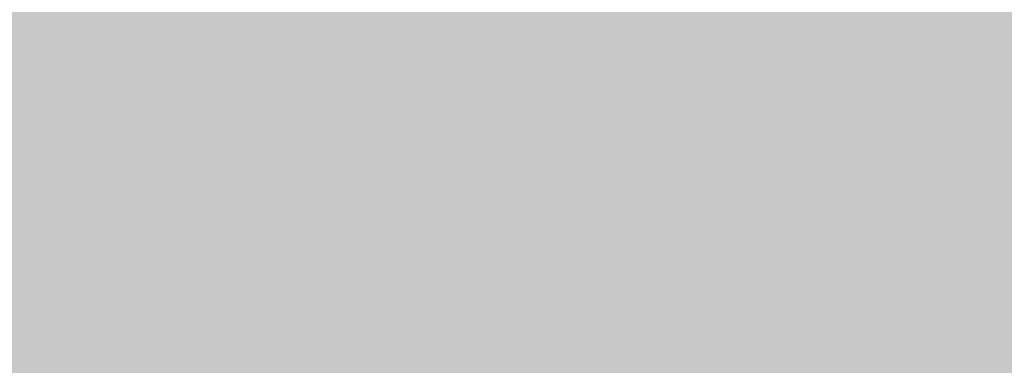
# Model space of a CAD drawing. Units: inches. Extents: x 2091 to 2899, y 967 to 2217.
# Tile 188 of 256: x 2203.16122 to 2203.18039, y 1152.25378 to 1152.26051. Entities that reach past the tile are written whole.
import ezdxf

# ---------------------------------------------------------------- set-up
doc = ezdxf.new("R2010")
doc.units = ezdxf.units.IN
doc.layers.add('A-WALL-PATT', color=141, linetype='Continuous', lineweight=13, true_color=0xadddf7)

msp = doc.modelspace()

# ---------------------------------------------------------------- hatches: boundary and pattern name
at = {"layer": 'A-WALL-PATT'}
h = msp.add_hatch(color=256, dxfattribs=at)
h.dxf.hatch_style = 1
h.paths.add_polyline_path([(2803.143603, 2050.919059), (2203.143603, 2050.919059), (2203.143603, 1090.919059), (2803.143603, 1090.919059)])
h.paths.add_polyline_path([(2635.79885, 1147.540465), (2674.524052, 1147.540465, 0.376086), (2678.529665, 1152.880202), (2678.529665, 1159.556473, 0.333335), (2674.524319, 1163.561846), (2674.524319, 1163.56185), (2674.524319, 1192.93439), (2635.805971, 1192.93439), (2597.087622, 1192.93439), (2597.087622, 1163.561846, 0.333335), (2593.082276, 1159.556473), (2593.082276, 1152.880202, 0.376086), (2597.087889, 1147.540465)], flags=0)
h.paths.add_polyline_path([(2436.010433, 1278.240778, 0.000483), (2435.952643, 1278.215027, -0.001328), (2435.935625, 1278.111693, -0.001711), (2436.11644, 1278.040758, 0.002185)], flags=0)
h.paths.add_polyline_path([(2794.143603, 1143.419059), (2794.143603, 1347.419059), (2543.370171, 1347.419059), (2543.370171, 1351.919059), (2794.143603, 1351.919059), (2794.143603, 1392.713555), (2793.947398, 1392.713555), (2793.947398, 1473.5369), (2794.143603, 1473.5369), (2794.143603, 1531.919059), (2650.143603, 1531.919059), (2650.143603, 1536.419059), (2794.143603, 1536.419059), (2794.143603, 1692.419059), (2609.375609, 1692.419059), (2609.375609, 1644.419059), (2604.875609, 1644.419059), (2604.875609, 1744.919059), (2609.375609, 1744.919059), (2609.375609, 1696.919059), (2794.143603, 1696.919059), (2794.143603, 1780.919059), (2609.643603, 1780.919059), (2493.875609, 1780.919059), (2493.875609, 1785.419059), (2609.643603, 1785.419059), (2794.143603, 1785.419059), (2794.143603, 1847.938821), (2793.951222, 1847.938821), (2793.951222, 1928.762166), (2794.143603, 1928.762166), (2794.143603, 1941.419059), (2614.143603, 1941.419059), (2614.143603, 1821.419059), (2609.643603, 1821.419059), (2609.643603, 1941.419059), (2392.143603, 1941.419059), (2392.143603, 1819.919059), (2387.643603, 1819.919059), (2387.643603, 1941.419059), (2212.143603, 1941.419059), (2212.143603, 1783.919059), (2392.143603, 1783.919059), (2392.143603, 1780.919059), (2212.143603, 1780.919059), (2212.143603, 1629.419059), (2387.643603, 1629.419059), (2387.643603, 1744.919059), (2392.143603, 1744.919059), (2392.143603, 1627.919059), (2317.143603, 1627.919059), (2317.143603, 1551.419059), (2317.143603, 1536.419059), (2459.383591, 1536.419059), (2459.383591, 1602.39648), (2463.883591, 1602.39648), (2463.883591, 1531.919059), (2456.643603, 1531.919059), (2456.643603, 1529.919059), (2452.143603, 1529.919059), (2452.143603, 1531.919059), (2312.643603, 1531.919059), (2312.643603, 1551.419059), (2306.143603, 1551.419059), (2306.143603, 1555.919059), (2308.143603, 1555.919059), (2308.143603, 1551.419059), (2312.643603, 1551.419059), (2312.643603, 1627.919059), (2212.143603, 1627.919059), (2212.143603, 1555.919059), (2270.143603, 1555.919059), (2270.143603, 1551.419059), (2212.143603, 1551.419059), (2212.143603, 1351.919059), (2272.143603, 1351.919059), (2272.143603, 1347.419059), (2212.143603, 1347.419059), (2212.143603, 1275.419059), (2308.143603, 1275.419059), (2308.143603, 1351.919059), (2452.143603, 1351.919059), (2452.143603, 1493.919059), (2456.643603, 1493.919059), (2456.643603, 1347.419059), (2312.643603, 1347.419059), (2312.643603, 1270.919059), (2212.143603, 1270.919059), (2212.143603, 1099.919059), (2281.237523, 1099.919059), (2282.871041, 1110.913803), (2282.008341, 1116.996603), (2278.557741, 1121.420403), (2268.205641, 1128.056203), (2272.087641, 1128.056203), (2273.812941, 1131.927003), (2279.420341, 1134.691903), (2285.027841, 1135.244903), (2287.615841, 1137.456803), (2288.047141, 1138.009803), (2289.341141, 1140.774703), (2291.066541, 1139.668703), (2292.360541, 1135.244903), (2295.379841, 1136.903803), (2296.242541, 1135.797903), (2297.105241, 1133.033003), (2300.124641, 1138.009803), (2303.143941, 1138.009803), (2304.437941, 1135.797903), (2303.143941, 1133.586003), (2306.594641, 1134.691903), (2307.888741, 1133.033003), (2310.908041, 1135.244903), (2313.927441, 1134.138903), (2315.62686, 1132.427102), (2308.320041, 1117.549603), (2290.203841, 1109.807903), (2288.909841, 1103.172103), (2289.272309, 1099.919059), (2434.918227, 1099.919059), (2431.593227, 1124.788059), (2429.930227, 1169.553059), (2430.927185, 1240.519694), (2435.658926, 1238.186126), (2437.135227, 1196.554059), (2438.798227, 1143.973059), (2442.678227, 1111.998059), (2446.558227, 1099.919059), (2794.143603, 1099.919059), (2794.143603, 1138.919059), (2548.032447, 1138.919059), (2548.032447, 1143.419059), (2548.032447, 1148.819059), (2546.668457, 1148.031559), (2528.685692, 1179.178622, 0.256256), (2512.032447, 1148.819059), (2512.032447, 1143.419059), (2512.032447, 1138.919059), (2507.532447, 1138.919059), (2507.532447, 1143.419059), (2507.532447, 1148.819059, 0.256256), (2490.879202, 1179.178622), (2472.896437, 1148.031559), (2471.532447, 1148.819059), (2471.532447, 1143.419059), (2467.032447, 1143.419059), (2467.032447, 1269.945786, 0.039061), (2460.909987, 1273.580059), (2467.032447, 1273.580059), (2467.032447, 1286.325364, 0.014511), (2465.216194, 1286.761905), (2467.032447, 1287.052576), (2467.032447, 1323.419059), (2471.532447, 1323.419059), (2471.532447, 1148.819059), (2489.532447, 1179.995973), (2490.896437, 1179.208473), (2490.879202, 1179.178622, -0.256256), (2507.532447, 1148.819059), (2507.532447, 1143.419059), (2512.032447, 1143.419059), (2512.032447, 1148.819059, -0.256256), (2528.685692, 1179.178622), (2528.668457, 1179.208473), (2530.032447, 1179.995973), (2548.032447, 1148.819059), (2548.032447, 1143.419059)], flags=16)
h.paths.add_polyline_path([(2607.768546, 1200.945083), (2607.768546, 1265.030625), (2597.087622, 1281.052011), (2619.784585, 1281.052011), (2627.795278, 1337.12686), (2635.79885, 1337.12686), (2643.816663, 1337.12686), (2651.827356, 1281.052011), (2674.524319, 1281.052011), (2663.843395, 1265.030625), (2663.843395, 1200.945083), (2635.805971, 1200.945083)], flags=0)
edge = h.paths.add_edge_path(flags=0)
edge.add_ellipse((13303.896215, 1272.998725), major_axis=(-10595.31304, 0.000001), ratio=0.842303870086, start_angle=0.6282372191, end_angle=0.6465540999, ccw=False)
edge.add_ellipse((2711.70045, 1156.852678), major_axis=(2.219769, 0), ratio=0.84230387, start_angle=111.535244, end_angle=180.628237, ccw=False)
edge.add_ellipse((13303.156292, 1272.998725), major_axis=(-10593.026306, 0), ratio=0.842303869544, start_angle=0.5282714718, end_angle=0.6465540971, ccw=False)
edge.add_line((2710.764596, 1175.333295), (2710.129986, 1175.333295))
edge.add_ellipse((2710.129986, 1176.579775), major_axis=(1.479846, 0), ratio=0.84230387, start_angle=180, end_angle=270, ccw=False)
edge.add_line((2708.65014, 1176.579775), (2708.65014, 1200.782914))
edge.add_ellipse((2710.129986, 1200.782914), major_axis=(1.479846, 0), ratio=0.84230387, start_angle=90, end_angle=180, ccw=False)
edge.add_line((2710.129986, 1202.029394), (2710.465075, 1202.029394))
edge.add_ellipse((13303.156292, 1272.998725), major_axis=(-10593.026306, 0), ratio=0.842303869544, start_angle=-0.0902290886, end_angle=0.3838667788, ccw=False)
edge.add_ellipse((2710.129986, 1290.927031), major_axis=(-1.479846, 0), ratio=0.84230387, start_angle=0, end_angle=90, ccw=False)
edge.add_line((2708.65014, 1290.927031), (2708.65014, 1315.13017))
edge.add_ellipse((2710.129986, 1315.13017), major_axis=(-1.479846, 0), ratio=0.84230387, start_angle=-90, end_angle=0, ccw=False)
edge.add_line((2710.129986, 1316.37665), (2710.706314, 1316.37665))
edge.add_ellipse((3238.40172, 1296.289566), major_axis=(528.234, 0), ratio=0.8423038695, start_angle=176.34957241, end_angle=177.82004969, ccw=False)
edge.add_ellipse((2775.063043, 1071.450696), major_axis=(313.307761, 0), ratio=0.8423038695, start_angle=102.12596555, end_angle=103.78052899, ccw=False)
edge.add_ellipse((2775.063043, 1078.305698), major_axis=(-305.302891, 0), ratio=0.8423038695, start_angle=-79.790461, end_angle=-77.55537271, ccw=False)
edge.add_ellipse((2695.141767, 1541.975383), major_axis=(-250.960216, 0), ratio=0.8423038695, start_angle=99.25656601, end_angle=102.55493264)
edge.add_line((2741.410326, 1334.214255), (2747.132545, 1337.378477))
edge.add_ellipse((2747.538616, 1336.857478), major_axis=(-0.739923, 0), ratio=0.8423039, start_angle=270, end_angle=307.93313, ccw=False)
edge.add_ellipse((2747.538616, 1336.857478), major_axis=(-0.739923, 0), ratio=0.8423039, start_angle=232.06687, end_angle=270, ccw=False)
edge.add_line((2747.944687, 1337.378477), (2753.666906, 1334.214255))
edge.add_ellipse((2799.935466, 1541.975383), major_axis=(250.960216, 0), ratio=0.8423038695, start_angle=257.44506736, end_angle=260.74343399)
edge.add_ellipse((2720.014189, 1078.305698), major_axis=(305.302891, 0), ratio=0.8423038695, start_angle=77.55537271, end_angle=79.790461, ccw=False)
edge.add_ellipse((2720.014189, 1071.450696), major_axis=(-313.307761, 0), ratio=0.8423038695, start_angle=256.21947101, end_angle=257.87403445, ccw=False)
edge.add_ellipse((2256.675512, 1296.289566), major_axis=(-528.234, 0), ratio=0.8423038695, start_angle=182.17995031, end_angle=183.65042759, ccw=False)
edge.add_line((2784.370918, 1316.37665), (2784.947247, 1316.37665))
edge.add_ellipse((2784.947247, 1315.13017), major_axis=(1.479846, 0), ratio=0.84230387, start_angle=0, end_angle=90, ccw=False)
edge.add_line((2786.427093, 1315.13017), (2786.427093, 1290.927031))
edge.add_ellipse((2784.947247, 1290.927031), major_axis=(1.479846, 0), ratio=0.84230387, start_angle=270, end_angle=360, ccw=False)
edge.add_ellipse((-7808.07906, 1272.998725), major_axis=(10593.026306, 0), ratio=0.842303869544, start_angle=-0.3838667788, end_angle=0.0902290886, ccw=False)
edge.add_line((2784.612157, 1202.029394), (2784.947247, 1202.029394))
edge.add_ellipse((2784.947247, 1200.782914), major_axis=(1.479846, 0), ratio=0.84230387, start_angle=0, end_angle=90, ccw=False)
edge.add_line((2786.427093, 1200.782914), (2786.427093, 1176.579775))
edge.add_ellipse((2784.947247, 1176.579775), major_axis=(-1.479846, 0), ratio=0.84230387, start_angle=90, end_angle=180, ccw=False)
edge.add_line((2784.947247, 1175.333295), (2784.312636, 1175.333295))
edge.add_ellipse((-7808.07906, 1272.998725), major_axis=(10593.026306, 0), ratio=0.842303869544, start_angle=-0.6186431963, end_angle=-0.5282714718, ccw=False)
edge.add_ellipse((2783.376783, 1156.852678), major_axis=(-2.219769, 0), ratio=0.84230387, start_angle=179.371763, end_angle=248.464757, ccw=False)
edge.add_ellipse((-7808.818983, 1272.998725), major_axis=(-10595.31304, 0.000004), ratio=0.842303865762, start_angle=179.3534459226, end_angle=179.3717628034, ccw=False)
edge.add_ellipse((2780.297303, 1153.500793), major_axis=(-5.246426, 0), ratio=0.84230387, start_angle=90, end_angle=179.353446, ccw=False)
edge.add_line((2780.297303, 1149.081708), (2714.77993, 1149.081708))
edge.add_ellipse((2714.77993, 1153.500793), major_axis=(5.246426, 0), ratio=0.84230387, start_angle=180.646554, end_angle=270, ccw=False)
edge = h.paths.add_edge_path(flags=0)
edge.add_line((2718.187367, 1151.007833), (2718.187367, 1170.472364))
edge.add_ellipse((2721.14706, 1170.472364), major_axis=(-2.959692, 0), ratio=0.84230387, start_angle=-90, end_angle=0, ccw=False)
edge.add_line((2721.14706, 1172.965324), (2773.930173, 1172.965324))
edge.add_ellipse((2773.930173, 1170.472364), major_axis=(-2.959692, 0), ratio=0.84230387, start_angle=180, end_angle=270, ccw=False)
edge.add_line((2776.889865, 1170.472364), (2776.889865, 1151.007833))
edge.add_line((2776.889865, 1151.007833), (2718.187367, 1151.007833))
edge = h.paths.add_edge_path(flags=0)
edge.add_line((2718.187367, 1180.23415), (2718.187367, 1199.057834))
edge.add_ellipse((2747.538616, 1320.39864), major_axis=(147.017924, 0), ratio=0.8423038695, start_angle=256.40186531, end_angle=283.59813469)
edge.add_line((2776.889865, 1199.057834), (2776.889865, 1180.23415))
edge.add_ellipse((2747.538616, 1301.574956), major_axis=(147.017924, 0), ratio=0.8423038695, start_angle=256.40186531, end_angle=283.59813469, ccw=False)
edge = h.paths.add_edge_path(flags=0)
edge.add_ellipse((13303.156292, 1272.998725), major_axis=(-10591.54646, 0), ratio=0.842303869555, start_angle=0.0555943135, end_angle=0.3777641939, ccw=False)
edge.add_line((2711.616859, 1262.72171), (2715.667408, 1249.495396))
edge.add_ellipse((6413.891963, 1241.691919), major_axis=(-3698.236159, 0), ratio=0.84230386955, start_angle=-0.120897369, end_angle=0.364076349)
edge.add_line((2715.761038, 1218.192455), (2711.934307, 1203.167361))
edge = h.paths.add_edge_path(flags=0)
edge.add_line((2718.187367, 1251.074566), (2716.002485, 1267.450435))
edge.add_ellipse((2742.151175, 1202.18954), major_axis=(81.772585, 0), ratio=0.84230387, start_angle=94.27742096, end_angle=111.8349538, ccw=False)
edge.add_line((2737.009748, 1270.930626), (2758.067484, 1270.930626))
edge.add_ellipse((2752.926058, 1202.18954), major_axis=(81.772585, 0), ratio=0.84230387, start_angle=68.1650462, end_angle=85.72257904, ccw=False)
edge.add_line((2779.074747, 1267.450435), (2776.889865, 1251.074566))
edge.add_ellipse((2750.338059, 1187.885356), major_axis=(79.579664, 0), ratio=0.84230387, start_angle=67.20808512, end_angle=85.1299304)
edge.add_line((2756.034656, 1254.743656), (2739.042576, 1254.743656))
edge.add_ellipse((2744.739174, 1187.885356), major_axis=(79.579664, 0), ratio=0.84230387, start_angle=94.8700696, end_angle=112.79191488)
edge = h.paths.add_edge_path(flags=0)
edge.add_line((2783.142926, 1203.167361), (2779.316194, 1218.192455))
edge.add_ellipse((-918.81473, 1241.691919), major_axis=(3698.236159, 0), ratio=0.84230386955, start_angle=-0.364076349, end_angle=0.120897369)
edge.add_line((2779.409825, 1249.495396), (2783.460373, 1262.72171))
edge.add_ellipse((-7808.07906, 1272.998725), major_axis=(-10591.54646, 0), ratio=0.84230386954, start_angle=179.6222358061, end_angle=179.9444056865, ccw=False)
edge = h.paths.add_edge_path(flags=0)
edge.add_ellipse((2734.200892, 1286.69044), major_axis=(-0.356609, 6.340078), ratio=0.60383358, start_angle=89.0020143, end_angle=253.657408, ccw=False)
edge.add_line((2730.369001, 1286.541806), (2730.369001, 1301.35198))
edge.add_line((2730.369001, 1301.35198), (2735.913311, 1305.214803))
edge.add_ellipse((2736.384917, 1304.734561), major_axis=(0.739923, 0), ratio=0.8423039, start_angle=90, end_angle=134.480211, ccw=False)
edge.add_line((2736.384917, 1305.357801), (2738.032783, 1305.357801))
edge.add_line((2738.032783, 1305.357801), (2738.032783, 1307.707927))
edge.add_ellipse((2794.201642, 1307.707927), major_axis=(56.168859, 0), ratio=0.84230387, start_angle=150.5614304, end_angle=180, ccw=False)
edge.add_ellipse((2700.875591, 1307.707927), major_axis=(-56.168859, 0), ratio=0.84230387, start_angle=180, end_angle=209.4385696, ccw=False)
edge.add_line((2757.04445, 1307.707927), (2757.04445, 1305.357801))
edge.add_line((2757.04445, 1305.357801), (2758.692316, 1305.357801))
edge.add_ellipse((2758.692316, 1304.734561), major_axis=(-0.739923, 0), ratio=0.8423039, start_angle=225.519789, end_angle=270, ccw=False)
edge.add_line((2759.163922, 1305.214803), (2764.708231, 1301.35198))
edge.add_line((2764.708231, 1301.35198), (2764.708231, 1286.541806))
edge.add_ellipse((2760.87634, 1286.69044), major_axis=(0.356609, 6.340078), ratio=0.60383358, start_angle=106.342592, end_angle=270.9979857, ccw=False)
edge.add_line((2757.04445, 1285.79709), (2757.04445, 1307.707927))
edge.add_ellipse((2700.875591, 1307.707927), major_axis=(-56.168859, 0), ratio=0.84230387, start_angle=180, end_angle=209.4385696)
edge.add_ellipse((2794.201642, 1307.707927), major_axis=(56.168859, 0), ratio=0.84230387, start_angle=150.5614304, end_angle=180)
edge.add_line((2738.032783, 1307.707927), (2738.032783, 1285.79709))
h.paths.add_polyline_path([(2417.812273, 1104.449704), (2413.492273, 1102.529704), (2410.612273, 1103.969704), (2409.172273, 1106.369704), (2407.252273, 1107.329704), (2406.292273, 1109.729704), (2405.332273, 1114.049704), (2405.332273, 1117.889704), (2406.292273, 1120.129704), (2407.252273, 1119.809704), (2408.848322, 1118.327658), (2410.173945, 1119.42417), (2410.211273, 1120.405704), (2411.040731, 1121.419054), (2410.699273, 1119.858704), (2410.173945, 1119.42417), (2410.088452, 1117.176109), (2411.132836, 1116.206324), (2413.972273, 1119.329704), (2416.852273, 1120.769704), (2416.869721, 1120.798784), (2417.035071, 1119.405116), (2417.896213, 1118.143384), (2418.292273, 1118.369704), (2419.544447, 1120.039269), (2419.360915, 1118.387487), (2419.032108, 1119.356151), (2418.398939, 1118.511926), (2419.252273, 1114.529704), (2418.794091, 1107.198795)], flags=0)
h.paths.add_polyline_path([(2508.870171, 1347.419059), (2508.370171, 1347.419059), (2508.370171, 1351.919059), (2508.870171, 1351.919059)], flags=0)
h.paths.add_polyline_path([(2473.370171, 1347.419059), (2472.370171, 1347.419059), (2467.870171, 1347.419059), (2467.870171, 1455.419059), (2472.370171, 1455.419059), (2472.370171, 1352.419059), (2473.370171, 1352.419059)], flags=0)
h.paths.add_polyline_path([(2352.106244, 1217.446197), (2349.226244, 1218.886197), (2347.786244, 1221.286197), (2345.866244, 1222.246197), (2344.906244, 1224.646197), (2343.946244, 1228.966197), (2343.946244, 1232.806197), (2344.906244, 1235.046197), (2345.866244, 1234.726197), (2347.462293, 1233.244152), (2348.787916, 1234.340663), (2348.825244, 1235.322197), (2349.654702, 1236.335547), (2349.313244, 1234.775197), (2348.787916, 1234.340663), (2348.702423, 1232.092603), (2349.746807, 1231.122817), (2352.586244, 1234.246197), (2355.466244, 1235.686197), (2355.483692, 1235.715277), (2355.649043, 1234.321609), (2356.510185, 1233.059877), (2356.906244, 1233.286197), (2358.158418, 1234.955762), (2357.974887, 1233.30398), (2357.646079, 1234.272644), (2357.012911, 1233.428419), (2357.866244, 1229.446197), (2357.408062, 1222.115288), (2356.426244, 1219.366197)], flags=0)
h.paths.add_polyline_path([(2348.2968, 1112.22442), (2347.0138, 1112.31042), (2345.5298, 1114.12742), (2345.7318, 1115.85842), (2346.8118, 1116.98242), (2346.8118, 1114.64642), (2345.8668, 1114.21442), (2346.8798, 1114.30042)], flags=0)
h.paths.add_polyline_path([(2347.0138, 1110.92642), (2346.2718, 1110.49342), (2346.6098, 1111.18642)], flags=0)
h.paths.add_polyline_path([(2345.8668, 1118.19442), (2345.5298, 1117.32942), (2343.7078, 1118.02142), (2344.3828, 1118.62642)], flags=0)
h.paths.add_polyline_path([(2346.6768, 1109.28242), (2346.0698, 1108.07142), (2345.8668, 1110.06142)], flags=0)
h.paths.add_polyline_path([(2345.0568, 1119.75142), (2343.6398, 1119.75142), (2343.9778, 1121.13542)], flags=0)
h.paths.add_polyline_path([(2345.2598, 1116.55042), (2345.1248, 1115.85842), (2344.9218, 1115.68542), (2344.7198, 1116.37742)], flags=0)
h.paths.add_polyline_path([(2345.6648, 1112.31042), (2345.4618, 1111.53242), (2344.0448, 1111.96442), (2344.6518, 1112.57042)], flags=0)
h.paths.add_polyline_path([(2345.1918, 1113.34942), (2344.4498, 1113.86842), (2344.7198, 1114.38742)], flags=0)
h.paths.add_polyline_path([(2344.6518, 1116.80942), (2344.1798, 1115.68542), (2344.6518, 1115.33942), (2343.9098, 1114.90642), (2343.0328, 1115.94442), (2343.6398, 1116.46342)], flags=0)
h.paths.add_polyline_path([(2345.8668, 1106.68642), (2344.9898, 1105.56242), (2344.5168, 1106.60042)], flags=0)
h.paths.add_polyline_path([(2344.8548, 1110.06142), (2344.5168, 1109.28242), (2344.1128, 1109.71542)], flags=0)
h.paths.add_polyline_path([(2344.0448, 1113.52242), (2343.4378, 1113.08942), (2342.7628, 1113.95442)], flags=0)
h.paths.add_polyline_path([(2344.3148, 1111.01242), (2342.9648, 1110.32042), (2342.9648, 1111.09942)], flags=0)
h.paths.add_polyline_path([(2345.1248, 1104.69742), (2344.5848, 1103.74542), (2344.4498, 1104.26442)], flags=0)
h.paths.add_polyline_path([(2342.8298, 1121.22242), (2341.7498, 1120.53042), (2340.5358, 1121.04942), (2340.1308, 1121.82842), (2340.6708, 1122.95242), (2341.1428, 1121.82842), (2341.6148, 1122.00142)], flags=0)
h.paths.add_polyline_path([(2342.9648, 1119.75142), (2343.0328, 1118.45342), (2342.0878, 1118.02142), (2342.0198, 1119.49142)], flags=0)
h.paths.add_polyline_path([(2342.6948, 1116.89642), (2341.9528, 1116.63642), (2342.0198, 1117.32942)], flags=0)
h.paths.add_polyline_path([(2343.0328, 1112.22442), (2342.0198, 1111.79142), (2341.5478, 1112.22442), (2342.3578, 1113.34942)], flags=0)
h.paths.add_polyline_path([(2343.7748, 1104.43742), (2342.6278, 1102.88042), (2342.6948, 1104.61042), (2343.4378, 1105.12942)], flags=0)
h.paths.add_polyline_path([(2342.0198, 1115.07942), (2340.8058, 1115.51242), (2340.9408, 1116.37742)], flags=0)
h.paths.add_polyline_path([(2341.4808, 1120.09742), (2341.4808, 1119.40542), (2341.0758, 1119.57842), (2341.1428, 1120.09742)], flags=0)
h.paths.add_polyline_path([(2341.8178, 1114.47342), (2340.9408, 1113.08942), (2340.8058, 1114.56042)], flags=0)
h.paths.add_polyline_path([(2341.1428, 1118.54042), (2340.9408, 1116.98242), (2339.0508, 1117.67542), (2339.0508, 1118.62642)], flags=0)
h.paths.add_polyline_path([(2342.6948, 1101.66842), (2341.9528, 1101.84142), (2342.5598, 1102.36142)], flags=0)
h.paths.add_polyline_path([(2340.3328, 1119.66542), (2338.4438, 1119.57842), (2337.9038, 1120.35742), (2339.6578, 1120.61642)], flags=0)
h.paths.add_polyline_path([(2340.3328, 1115.33942), (2340.0628, 1113.69542), (2339.3878, 1115.33942)], flags=0)
h.paths.add_polyline_path([(2341.8178, 1103.83142), (2341.5478, 1102.88042), (2341.1428, 1103.65842)], flags=0)
h.paths.add_polyline_path([(2339.0508, 1122.86642), (2337.2958, 1121.82842), (2337.0938, 1123.12542), (2337.7688, 1123.81842)], flags=0)
h.paths.add_polyline_path([(2339.1178, 1121.74142), (2338.8478, 1121.22242), (2338.1738, 1121.04942), (2338.3758, 1121.56842)], flags=0)
h.paths.add_polyline_path([(2339.1858, 1119.31942), (2338.6458, 1118.71342), (2338.2408, 1118.10742), (2338.2408, 1118.88642)], flags=0)
h.paths.add_polyline_path([(2341.1428, 1101.92842), (2340.6028, 1101.23642), (2340.0628, 1101.84142), (2340.6028, 1102.36142)], flags=0)
h.paths.add_polyline_path([(2337.6338, 1117.76142), (2336.6208, 1118.28042), (2337.2958, 1118.97242)], flags=0)
h.paths.add_polyline_path([(2336.8238, 1119.57842), (2334.7988, 1118.97242), (2335.2038, 1120.35742), (2336.5538, 1120.87642)], flags=0)
h.paths.add_polyline_path([(2339.1178, 1100.45742), (2337.3638, 1100.54342), (2336.7558, 1101.23642)], flags=0)
h.paths.add_polyline_path([(2336.3508, 1122.43342), (2336.0138, 1121.91442), (2334.9338, 1122.43342), (2334.5288, 1123.47142), (2335.7438, 1122.77942)], flags=0)
h.paths.add_polyline_path([(2334.7318, 1120.87642), (2334.2588, 1120.35742), (2334.0568, 1120.78942), (2334.5968, 1121.30842)], flags=0)
h.paths.add_polyline_path([(2334.4618, 1122.17442), (2332.5718, 1121.30842), (2331.3568, 1122.17442), (2332.0998, 1122.86642)], flags=0)
h.paths.add_polyline_path([(2334.2588, 1118.54042), (2333.3818, 1118.45342), (2333.6518, 1119.31942)], flags=0)
h.paths.add_polyline_path([(2335.5418, 1102.27442), (2334.1918, 1102.62042), (2335.2718, 1103.31242)], flags=0)
h.paths.add_polyline_path([(2332.7068, 1119.66542), (2331.6948, 1120.44342), (2332.5048, 1120.78942)], flags=0)
h.paths.add_polyline_path([(2334.7318, 1101.14942), (2333.5168, 1101.58242), (2333.9888, 1101.75542)], flags=0)
h.paths.add_polyline_path([(2332.6398, 1116.63642), (2331.0868, 1116.29042), (2331.9648, 1118.19442)], flags=0)
h.paths.add_polyline_path([(2330.7498, 1121.56842), (2330.2768, 1120.27042), (2328.5228, 1119.31942), (2328.9948, 1121.04942)], flags=0)
h.paths.add_polyline_path([(2330.7498, 1118.62642), (2330.0078, 1117.50242), (2329.8728, 1118.02142)], flags=0)
h.paths.add_polyline_path([(2332.0998, 1102.36142), (2330.5468, 1102.01442), (2331.6948, 1102.96642)], flags=0)
h.paths.add_polyline_path([(2329.5348, 1113.60842), (2329.0628, 1112.31042), (2328.5898, 1113.34942)], flags=0)
h.paths.add_polyline_path([(2328.3878, 1117.84842), (2327.5098, 1116.55042), (2327.1728, 1117.76142)], flags=0)
h.paths.add_polyline_path([(2329.7378, 1106.51342), (2329.5348, 1105.30242), (2328.2528, 1106.08142)], flags=0)
h.paths.add_polyline_path([(2328.6578, 1114.38742), (2328.0498, 1114.12742), (2328.3198, 1114.90642)], flags=0)
h.paths.add_polyline_path([(2328.3198, 1112.22442), (2327.1058, 1112.13742), (2326.7008, 1112.65642)], flags=0)
h.paths.add_polyline_path([(2326.9028, 1115.25242), (2326.7008, 1114.12742), (2325.2158, 1113.60842), (2326.0928, 1115.33942)], flags=0)
h.paths.add_polyline_path([(2326.6328, 1108.33042), (2326.0928, 1107.37942), (2325.8908, 1108.50342), (2326.4978, 1109.10942)], flags=0)
h.paths.add_polyline_path([(2615.143603, 1531.919059), (2609.643603, 1531.919059), (2609.643603, 1620.419059), (2614.143603, 1620.419059), (2614.143603, 1536.419059), (2615.143603, 1536.419059)], flags=0)
h.paths.add_polyline_path([(2545.143603, 1563.419059), (2464.143603, 1563.419059), (2464.143603, 1632.419059), (2509.143603, 1632.419059), (2509.143603, 1627.919059), (2509.143603, 1603.919059), (2468.643603, 1603.919059), (2468.643603, 1567.919059), (2540.643603, 1567.919059), (2540.643603, 1591.919059), (2545.143603, 1591.919059)], flags=0)
h.paths.add_polyline_path([(2388.969048, 1549.985735), (2357.434181, 1549.985735), (2357.434181, 1623.360778), (2399.362777, 1623.360778), (2435.689465, 1623.360778), (2435.592547, 1602.559273), (2435.592547, 1602.39648), (2388.969048, 1602.39648)], flags=0)
h.paths.add_polyline_path([(2388.880628, 1555.809151), (2374.904429, 1555.809151), (2374.904429, 1600.571564), (2374.904429, 1615.457645), (2406.350877, 1615.457645), (2406.350877, 1618.939431), (2412.174293, 1615.457645), (2406.350877, 1611.97586), (2406.350877, 1615.457645), (2388.880628, 1615.457645)], flags=0)
h.paths.add_polyline_path([(2568.875609, 1644.419059), (2453.375609, 1644.419059), (2453.375609, 1785.419059), (2457.875609, 1785.419059), (2457.875609, 1648.919059), (2568.875609, 1648.919059)], flags=0)
h.paths.add_polyline_path([(2212.143603, 1945.919059), (2212.143603, 2041.919059), (2794.143603, 2041.919059), (2794.143603, 1945.919059)], flags=16)
h.paths.add_polyline_path([(2271.082728, 1964.317238), (2776.852968, 1964.317238), (2776.852968, 2037.169623), (2271.082728, 2037.169623)], flags=8)
h.paths.add_polyline_path([(2380.649285, 1536.824144), (2461.040809, 1536.824144), (2461.040809, 1554.652587), (2380.649285, 1554.652587)], flags=8)
h.paths.add_polyline_path([(2240.755709, 1609.725451), (2309.185829, 1609.725451), (2309.185829, 1617.698204), (2240.755709, 1617.698204)], flags=8)
h.paths.add_polyline_path([(2212.677255, 1313.504102), (2282.59152, 1313.504102), (2282.59152, 1322.745239), (2212.677255, 1322.745239)], flags=8)
h.paths.add_polyline_path([(2457.111976, 1114.778574), (2558.481581, 1114.778574), (2558.481581, 1142.219682), (2457.111976, 1142.219682)], flags=8)
h.paths.add_polyline_path([(2473.442337, 1273.010067), (2604.641226, 1273.010067), (2604.641226, 1318.346935), (2473.442337, 1318.346935)], flags=8)
h.paths.add_polyline_path([(2638.876302, 1626.977432), (2684.250367, 1627.976738), (2684.038483, 1637.597494), (2638.664417, 1636.598188)], flags=8)
h.paths.add_polyline_path([(2537.590554, 1453.793447), (2628.389547, 1453.793447), (2628.389547, 1475.344811), (2537.590554, 1475.344811)], flags=8)
h.paths.add_polyline_path([(2504.137638, 1714.632397), (2554.647187, 1714.632397), (2554.647187, 1730.237712), (2504.137638, 1730.237712)], flags=8)
h.paths.add_polyline_path([(2487.501181, 1575.651872), (2535.097121, 1575.651872), (2535.097121, 1598.377646), (2487.501181, 1598.377646)], flags=8)
h.paths.add_polyline_path([(2709.0994, 1735.710278), (2740.016601, 1735.710278), (2740.016601, 1749.937641), (2709.0994, 1749.937641)], flags=8)
h.paths.add_polyline_path([(2442.438424, 1792.171657), (2564.728835, 1792.171657), (2564.728835, 1842.000163), (2442.438424, 1842.000163)], flags=8)
h.paths.add_polyline_path([(2655.815801, 1809.644076), (2789.520142, 1806.693796), (2790.084977, 1832.291638), (2656.380635, 1835.241918)], flags=8)
h.paths.add_polyline_path([(2234.842697, 1797.720143), (2368.592851, 1794.768852), (2369.160718, 1820.504132), (2235.410564, 1823.455423)], flags=8)
h.paths.add_polyline_path([(2245.138466, 1644.006335), (2398.427733, 1640.6239), (2398.994842, 1666.32482), (2245.705575, 1669.707255)], flags=8)
h.paths.add_polyline_path([(2306.142847, 1431.168519), (2413.768314, 1428.793687), (2414.333148, 1454.391529), (2306.707682, 1456.76636)], flags=8)
h.paths.add_polyline_path([(2306.834582, 1458.233145), (2393.380484, 1456.323449), (2393.932808, 1481.354358), (2307.386907, 1483.264054)], flags=8)

doc.saveas('drawing.dxf')
